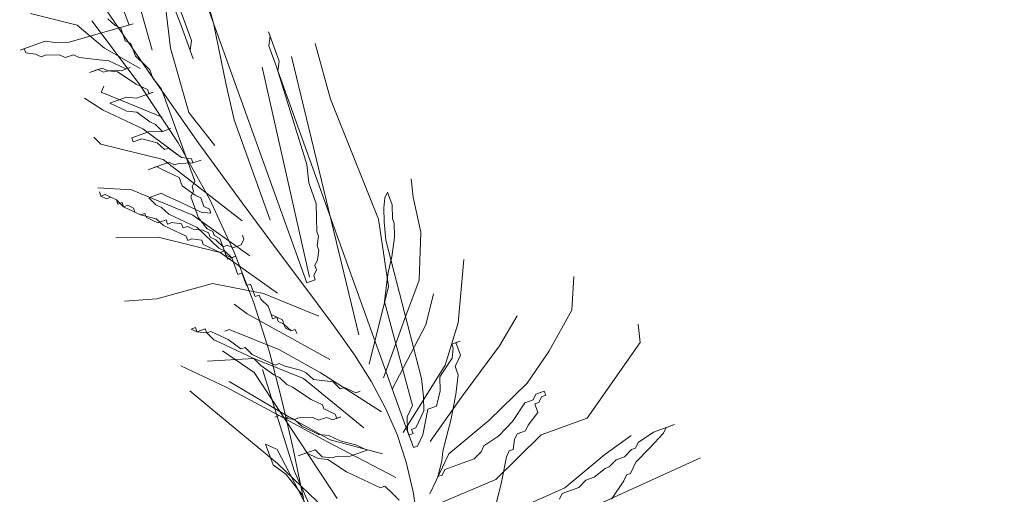
# Model space of a CAD drawing. Units: millimetres. Extents: x 595116 to 630915, y 909473 to 920225.
# Tile 38 of 134: x 629665.643 to 629671.98, y 919177.461 to 919180.516. Entities that reach past the tile are written whole.
import ezdxf

# ---------------------------------------------------------------- set-up
doc = ezdxf.new("R2010")
doc.units = ezdxf.units.MM
doc.layers.add('Dimension', color=3, linetype='Continuous', lineweight=18)
doc.layers.add('L-PLNT', color=85, linetype='Continuous', lineweight=13)
doc.styles.get("Standard").update_dxf_attribs({"font": 'arial.ttf'})
doc.dimstyles.new('ISO-25', dxfattribs={"dimtxt": 9, "dimasz": 6, "dimexe": 1.25, "dimexo": 0.625, "dimtad": 1, "dimlunit": 4, "dimtxsty": 'Standard', "dimcen": 2.5, "dimadec": 0, "dimazin": 0, "dimtfac": 1, "dimtmove": 0, "dimatfit": 3, "dimfxl": 1, "dimarcsym": 0})

# ---------------------------------------------------------------- blocks, each defined once
blk = doc.blocks.new('A$C4FB75ABC')
for p, q in [((2.6279, 3.8295), (2.3336, 4.6475)), ((2.4125, 4.2707), (2.3227, 4.4977)), ((2.3232, 4.271), (2.2922, 4.3571)), ((2.4678, 4.2744), (2.4414, 4.3703)), ((2.2538, 4.3417), (2.3557, 4.1924)), ((2.3628, 4.2285), (2.3338, 4.3316)), ((2.3941, 4.2317), (2.382, 4.3327)), ((2.234, 4.2713), (2.154, 4.2911)), ((2.4119, 4.2948), (2.43, 4.2446)), ((2.2202, 4.242), (2.3304, 4.2736)), ((2.2808, 4.2314), (2.234, 4.2713)), ((2.3407, 4.1707), (2.2593, 4.2788)), ((2.2868, 4.2822), (2.2991, 4.2704)), ((2.4896, 4.1688), (2.4678, 4.2744)), ((2.2991, 4.2704), (2.3089, 4.2658)), ((2.3089, 4.2658), (2.3166, 4.2443)), ((2.4331, 4.2133), (2.4125, 4.2707)), ((2.5803, 4.2095), (2.5622, 4.2597)), ((2.5622, 4.2597), (2.5648, 4.2526)), ((2.1362, 4.228), (2.1792, 4.2435)), ((2.1792, 4.2435), (2.1961, 4.2415)), ((2.1961, 4.2415), (2.2202, 4.242)), ((2.3166, 4.2443), (2.3264, 4.2397)), ((2.3264, 4.2397), (2.3341, 4.2182)), ((2.43, 4.2446), (2.4279, 4.2276)), ((2.5648, 4.2526), (2.5628, 4.2356)), ((2.6686, 4.144), (2.6423, 4.2399)), ((2.1434, 4.2306), (2.1362, 4.228)), ((2.1459, 4.2234), (2.1434, 4.2306)), ((2.1629, 4.2214), (2.1459, 4.2234)), ((2.1726, 4.2168), (2.1629, 4.2214)), ((2.3419, 4.1967), (2.2808, 4.2314)), ((2.4257, 4.1214), (2.3941, 4.2317)), ((2.4279, 4.2276), (2.4331, 4.2133)), ((2.5628, 4.2356), (2.5757, 4.1997)), ((2.1798, 4.2194), (2.1726, 4.2168)), ((2.2039, 4.22), (2.1798, 4.2194)), ((2.2136, 4.2154), (2.2039, 4.22)), ((2.228, 4.2205), (2.2136, 4.2154)), ((2.2377, 4.2159), (2.228, 4.2205)), ((2.2716, 4.2119), (2.2377, 4.2159)), ((2.2885, 4.2099), (2.2716, 4.2119)), ((2.308, 4.2007), (2.2885, 4.2099)), ((2.3341, 4.2182), (2.3465, 4.2064)), ((2.3465, 4.2064), (2.3588, 4.1946)), ((2.5783, 4.1926), (2.5803, 4.2095)), ((2.7169, 3.7399), (2.6018, 4.2172)), ((2.2552, 4.1898), (2.2768, 4.1975)), ((2.2696, 4.195), (2.2552, 4.1898)), ((2.2793, 4.1904), (2.2696, 4.195)), ((2.2768, 4.1975), (2.2865, 4.1929)), ((2.2865, 4.1929), (2.2793, 4.1904)), ((2.2865, 4.1929), (2.3106, 4.1935)), ((2.3034, 4.1909), (2.2865, 4.1929)), ((2.3353, 4.17), (2.3034, 4.1909)), ((2.3178, 4.1961), (2.308, 4.2007)), ((2.3106, 4.1935), (2.325, 4.1987)), ((2.325, 4.1987), (2.3178, 4.1961)), ((2.3557, 4.1924), (2.443, 4.0685)), ((2.3588, 4.1946), (2.364, 4.1803)), ((2.6325, 3.8393), (2.5516, 4.1992)), ((2.5757, 4.1997), (2.6279, 4.0321)), ((2.8029, 3.5683), (2.5783, 4.1926)), ((2.345, 4.1654), (2.3353, 4.17)), ((2.4072, 4.0691), (2.3407, 4.1707)), ((2.364, 4.1803), (2.3789, 4.1614)), ((2.2753, 4.1565), (2.2799, 4.1663)), ((2.38, 4.1131), (2.2753, 4.1565)), ((2.3359, 4.1459), (2.3645, 4.1562)), ((2.3548, 4.1608), (2.345, 4.1654)), ((2.3574, 4.1536), (2.3548, 4.1608)), ((2.3645, 4.1562), (2.3574, 4.1536)), ((2.3789, 4.1614), (2.4357, 4.0035)), ((2.5031, 4.1088), (2.4896, 4.1688)), ((2.2785, 4.1252), (2.2466, 4.1462)), ((2.2902, 4.1376), (2.3189, 4.1479)), ((2.3, 4.133), (2.2902, 4.1376)), ((2.3189, 4.1479), (2.3359, 4.1459)), ((2.7507, 3.9385), (2.6686, 4.144)), ((2.3468, 4.0931), (2.2785, 4.1252)), ((2.3098, 4.1284), (2.3, 4.133)), ((2.3195, 4.1238), (2.3098, 4.1284)), ((2.3364, 4.1218), (2.3195, 4.1238)), ((2.3585, 4.1054), (2.3364, 4.1218)), ((2.4704, 4.0646), (2.4257, 4.1214)), ((2.3683, 4.1008), (2.3585, 4.1054)), ((2.5651, 3.9366), (2.5031, 4.1088)), ((2.3278, 4.0781), (2.3565, 4.0885)), ((2.413, 4.044), (2.3468, 4.0931)), ((2.3565, 4.0885), (2.3806, 4.089)), ((2.3806, 4.089), (2.3683, 4.1008)), ((2.3806, 4.089), (2.395, 4.0942)), ((2.395, 4.0942), (2.3806, 4.089)), ((2.275, 4.0672), (2.2627, 4.079)), ((2.3304, 4.071), (2.3278, 4.0781)), ((2.3448, 4.0761), (2.3304, 4.071)), ((2.3714, 4.0695), (2.3448, 4.0761)), ((2.3838, 4.0577), (2.3714, 4.0695)), ((2.4608, 3.9732), (2.4072, 4.0691)), ((2.3818, 4.0408), (2.275, 4.0672)), ((2.3909, 4.0603), (2.3838, 4.0577)), ((2.413, 4.044), (2.3909, 4.0603)), ((2.443, 4.0685), (2.5171, 3.9664)), ((2.3557, 4.0233), (2.3915, 4.0362)), ((2.5169, 3.9354), (2.3818, 4.0408)), ((2.3915, 4.0362), (2.4013, 4.0316)), ((2.43, 4.0419), (2.413, 4.044)), ((2.4325, 4.0348), (2.43, 4.0419)), ((2.4325, 4.0348), (2.4469, 4.0399)), ((2.4469, 4.0399), (2.4325, 4.0348)), ((2.37, 4.0285), (2.3557, 4.0233)), ((2.3798, 4.0239), (2.37, 4.0285)), ((2.3993, 4.0147), (2.3798, 4.0239)), ((2.4013, 4.0316), (2.4084, 4.0342)), ((2.4084, 4.0342), (2.4325, 4.0348)), ((2.6279, 4.0321), (2.6311, 4.0008)), ((2.409, 4.0101), (2.3993, 4.0147)), ((2.4142, 3.9957), (2.409, 4.0101)), ((2.4357, 4.0035), (2.4311, 3.9937)), ((2.8101, 3.9761), (2.8069, 4.0074)), ((2.3275, 3.9889), (2.2696, 3.9923)), ((2.2748, 3.978), (2.2722, 3.9852)), ((2.2722, 3.9852), (2.2748, 3.978)), ((2.4323, 3.9455), (2.3275, 3.9889)), ((2.4363, 3.9794), (2.4142, 3.9957)), ((2.4337, 3.9866), (2.4291, 3.9768)), ((2.4311, 3.9937), (2.4337, 3.9866)), ((2.6311, 4.0008), (2.644, 3.965)), ((2.7665, 3.9847), (2.7619, 3.975)), ((2.7742, 3.9632), (2.7665, 3.9847)), ((2.2748, 3.978), (2.2819, 3.9806)), ((2.2845, 3.9734), (2.2748, 3.978)), ((2.2819, 3.9806), (2.2917, 3.976)), ((2.2917, 3.976), (2.2845, 3.9734)), ((2.3014, 3.9714), (2.2917, 3.976)), ((2.2917, 3.976), (2.3014, 3.9714)), ((2.304, 3.9642), (2.3014, 3.9714)), ((2.3014, 3.9714), (2.3138, 3.9596)), ((2.3568, 3.9751), (2.3783, 3.9828)), ((2.3691, 3.9633), (2.3568, 3.9751)), ((2.3783, 3.9828), (2.3881, 3.9782)), ((2.3881, 3.9782), (2.4076, 3.9691)), ((2.4076, 3.9691), (2.4173, 3.9645)), ((2.4291, 3.9768), (2.442, 3.9409)), ((2.446, 3.9748), (2.4363, 3.9794)), ((2.4512, 3.9604), (2.446, 3.9748)), ((2.5035, 3.8821), (2.4608, 3.9732)), ((2.7619, 3.975), (2.7599, 3.958)), ((2.8236, 3.9161), (2.8101, 3.9761)), ((2.3112, 3.9668), (2.304, 3.9642)), ((2.3138, 3.9596), (2.3112, 3.9668)), ((2.3209, 3.9622), (2.3138, 3.9596)), ((2.3138, 3.9596), (2.3235, 3.955)), ((2.3307, 3.9576), (2.3209, 3.9622)), ((2.3235, 3.955), (2.3333, 3.9504)), ((2.3333, 3.9504), (2.3307, 3.9576)), ((2.3789, 3.9587), (2.3691, 3.9633)), ((2.3912, 3.947), (2.3789, 3.9587)), ((2.4173, 3.9645), (2.4368, 3.9553)), ((2.4368, 3.9553), (2.4466, 3.9507)), ((2.4466, 3.9507), (2.4635, 3.9487)), ((2.4609, 3.9558), (2.4512, 3.9604)), ((2.4635, 3.9487), (2.4609, 3.9558)), ((2.5171, 3.9664), (2.5794, 3.8826)), ((2.644, 3.965), (2.6451, 3.9167)), ((2.7599, 3.958), (2.7605, 3.9339)), ((2.7748, 3.9391), (2.7742, 3.9632)), ((2.343, 3.9458), (2.3333, 3.9504)), ((2.3333, 3.9504), (2.343, 3.9458)), ((2.3502, 3.9484), (2.343, 3.9458)), ((2.343, 3.9458), (2.3697, 3.9392)), ((2.3528, 3.9412), (2.3502, 3.9484)), ((2.3723, 3.932), (2.3528, 3.9412)), ((2.3697, 3.9392), (2.3821, 3.9274)), ((2.3866, 3.9372), (2.3723, 3.932)), ((2.3892, 3.93), (2.3866, 3.9372)), ((2.401, 3.9424), (2.3912, 3.947)), ((2.44, 3.924), (2.401, 3.9424)), ((2.5304, 3.8755), (2.4323, 3.9455)), ((2.442, 3.9409), (2.4569, 3.922)), ((2.7679, 3.8231), (2.7507, 3.9385)), ((2.7605, 3.9339), (2.7636, 3.9026)), ((2.7774, 3.9319), (2.7748, 3.9391)), ((2.3821, 3.9274), (2.3918, 3.9228)), ((2.3964, 3.9326), (2.3892, 3.93)), ((2.3918, 3.9228), (2.4113, 3.9137)), ((2.4133, 3.9306), (2.3964, 3.9326)), ((2.4159, 3.9234), (2.4133, 3.9306)), ((2.4231, 3.926), (2.4159, 3.9234)), ((2.4328, 3.9214), (2.4231, 3.926)), ((2.4498, 3.9194), (2.4328, 3.9214)), ((2.4523, 3.9122), (2.44, 3.924)), ((2.4595, 3.9148), (2.4498, 3.9194)), ((2.4569, 3.922), (2.4667, 3.9174)), ((2.4667, 3.9174), (2.4693, 3.9102)), ((2.6451, 3.9167), (2.6477, 3.9096)), ((2.778, 3.9078), (2.7774, 3.9319)), ((2.3729, 3.9079), (2.3006, 3.9062)), ((2.4796, 3.8815), (2.3729, 3.9079)), ((2.4113, 3.9137), (2.4211, 3.9091)), ((2.4211, 3.9091), (2.4237, 3.9019)), ((2.4237, 3.9019), (2.4308, 3.9045)), ((2.4308, 3.9045), (2.4478, 3.9025)), ((2.4478, 3.9025), (2.4503, 3.8953)), ((2.477, 3.8887), (2.4523, 3.9122)), ((2.4621, 3.9076), (2.4595, 3.9148)), ((2.4718, 3.903), (2.4621, 3.9076)), ((2.4693, 3.9102), (2.479, 3.9056)), ((2.4842, 3.8913), (2.4718, 3.903)), ((2.479, 3.9056), (2.4868, 3.8841)), ((2.52, 3.9042), (2.5155, 3.8944)), ((2.5175, 3.9113), (2.52, 3.9042)), ((2.6477, 3.9096), (2.6457, 3.8926)), ((2.7636, 3.9026), (2.8247, 3.6653)), ((2.7739, 3.8739), (2.778, 3.9078)), ((2.8207, 3.834), (2.8236, 3.9161)), ((2.4503, 3.8953), (2.4698, 3.8861)), ((2.4698, 3.8861), (2.4796, 3.8815)), ((2.4868, 3.8841), (2.477, 3.8887)), ((2.4796, 3.8815), (2.4868, 3.8841)), ((2.4914, 3.8938), (2.4842, 3.8913)), ((2.4868, 3.8841), (2.4893, 3.8769)), ((2.4919, 3.8697), (2.4868, 3.8841)), ((2.4868, 3.8841), (2.4991, 3.8723)), ((2.5011, 3.8892), (2.4914, 3.8938)), ((2.5155, 3.8944), (2.5011, 3.8892)), ((2.6457, 3.8926), (2.6483, 3.8855)), ((2.6483, 3.8855), (2.6463, 3.8685)), ((2.5777, 3.8114), (2.4796, 3.8815)), ((2.4893, 3.8769), (2.4991, 3.8723)), ((2.5063, 3.8749), (2.4919, 3.8697)), ((2.4991, 3.8723), (2.5063, 3.8749)), ((2.4991, 3.8723), (2.5094, 3.8436)), ((2.5372, 3.7949), (2.5035, 3.8821)), ((2.5794, 3.8826), (2.6314, 3.8136)), ((2.6463, 3.8685), (2.6417, 3.8588)), ((2.7673, 3.8473), (2.7739, 3.8739)), ((2.8876, 3.7608), (2.897, 3.8696)), ((2.6443, 3.8516), (2.6397, 3.8418)), ((2.6417, 3.8588), (2.6443, 3.8516)), ((2.5094, 3.8436), (2.5166, 3.8462)), ((2.5166, 3.8462), (2.5244, 3.8247)), ((2.6423, 3.8347), (2.6279, 3.8295)), ((2.6397, 3.8418), (2.6423, 3.8347)), ((2.7653, 3.8303), (2.7673, 3.8473)), ((2.7957, 3.7683), (2.8207, 3.834)), ((3.0823, 3.7823), (3.0858, 3.8403)), ((2.4664, 3.8281), (2.3706, 3.8017)), ((2.5536, 3.8109), (2.4664, 3.8281)), ((2.5244, 3.8247), (2.5315, 3.8272)), ((2.5315, 3.8272), (2.5393, 3.8057)), ((2.7349, 3.6897), (2.7679, 3.8231)), ((2.7613, 3.7965), (2.7653, 3.8303)), ((2.3706, 3.8017), (2.3152, 3.798)), ((2.5393, 3.8057), (2.5464, 3.8083)), ((2.5464, 3.8083), (2.549, 3.8011)), ((2.549, 3.8011), (2.5614, 3.7893)), ((2.6486, 3.7721), (2.5536, 3.8109)), ((2.6314, 3.8136), (2.6743, 3.7558)), ((2.8322, 3.7571), (2.8454, 3.8105)), ((2.5255, 3.7764), (2.5034, 3.7928)), ((2.5638, 3.7106), (2.5372, 3.7949)), ((2.5614, 3.7893), (2.5665, 3.775)), ((2.8089, 3.6191), (2.7613, 3.7965)), ((3.043, 3.7114), (3.0823, 3.7823)), ((2.6672, 3.6978), (2.5255, 3.7764)), ((2.5665, 3.775), (2.5763, 3.7704)), ((2.5691, 3.7678), (2.5665, 3.775)), ((2.5763, 3.7704), (2.5691, 3.7678)), ((2.5763, 3.7704), (2.5789, 3.7632)), ((2.586, 3.7658), (2.5763, 3.7704)), ((2.5886, 3.7586), (2.586, 3.7658)), ((2.7596, 3.6662), (2.7957, 3.7683)), ((2.9584, 3.7215), (2.9885, 3.7729)), ((2.4369, 3.7526), (2.4297, 3.7501)), ((2.4297, 3.7501), (2.4394, 3.7455)), ((2.4394, 3.7455), (2.4369, 3.7526)), ((2.4538, 3.7506), (2.4394, 3.7455)), ((2.4564, 3.7435), (2.4538, 3.7506)), ((2.4948, 3.7492), (2.4876, 3.7466)), ((2.58, 3.715), (2.4948, 3.7492)), ((2.5789, 3.7632), (2.5886, 3.7586)), ((2.5886, 3.7586), (2.5912, 3.7515)), ((2.601, 3.7469), (2.5886, 3.7586)), ((2.5912, 3.7515), (2.601, 3.7469)), ((2.601, 3.7469), (2.6081, 3.7494)), ((2.6081, 3.7494), (2.601, 3.7469)), ((2.6081, 3.7494), (2.6107, 3.7423)), ((2.6107, 3.7423), (2.6081, 3.7494)), ((2.6743, 3.7558), (2.7096, 3.7056)), ((2.7745, 3.6472), (2.8322, 3.7571)), ((2.8652, 3.6879), (2.8876, 3.7608)), ((3.1994, 3.7272), (3.1962, 3.7584)), ((2.4394, 3.7455), (2.4564, 3.7435)), ((2.4635, 3.746), (2.4564, 3.7435)), ((2.4564, 3.7435), (2.4687, 3.7317)), ((2.4733, 3.7414), (2.4635, 3.746)), ((2.4687, 3.7317), (2.4785, 3.7271)), ((2.4928, 3.7323), (2.4733, 3.7414)), ((2.5149, 3.7159), (2.4928, 3.7323)), ((2.4785, 3.7271), (2.498, 3.7179)), ((2.498, 3.7179), (2.5272, 3.7041)), ((2.5221, 3.7185), (2.5149, 3.7159)), ((2.5344, 3.7067), (2.5221, 3.7185)), ((2.6509, 3.6757), (2.58, 3.715)), ((2.8907, 3.7295), (2.8764, 3.7244)), ((2.8764, 3.7244), (2.8789, 3.7172)), ((2.8789, 3.7172), (2.8769, 3.7003)), ((2.8835, 3.727), (2.8907, 3.7295)), ((2.8913, 3.7054), (2.8835, 3.727)), ((2.893, 3.6331), (2.9584, 3.7215)), ((3.1085, 3.5972), (3.1994, 3.7272)), ((2.537, 3.6995), (2.4575, 3.6952)), ((2.5376, 3.6754), (2.4836, 3.7127)), ((2.5272, 3.7041), (2.537, 3.6995)), ((2.5441, 3.7021), (2.5344, 3.7067)), ((2.537, 3.6995), (2.5493, 3.6877)), ((2.6222, 3.6653), (2.537, 3.6995)), ((2.5637, 3.6929), (2.5441, 3.7021)), ((2.5853, 3.6284), (2.5638, 3.7106)), ((2.7096, 3.7056), (2.7388, 3.6597)), ((2.8769, 3.7003), (2.856, 3.6684)), ((2.8821, 3.6859), (2.8913, 3.7054)), ((3.0058, 3.6575), (3.043, 3.7114)), ((2.4899, 3.6502), (2.4119, 3.6869)), ((2.5493, 3.6877), (2.5714, 3.6714)), ((2.6067, 3.5058), (2.5519, 3.6806)), ((2.5734, 3.6883), (2.5637, 3.6929)), ((2.5806, 3.6909), (2.5734, 3.6883)), ((2.5903, 3.6863), (2.5806, 3.6909)), ((2.617, 3.6797), (2.5903, 3.6863)), ((2.7932, 3.5729), (2.8652, 3.6879)), ((2.8873, 3.6716), (2.8821, 3.6859)), ((2.6801, 3.4593), (2.5376, 3.6754)), ((2.5714, 3.6714), (2.5812, 3.6668)), ((2.5812, 3.6668), (2.5935, 3.655)), ((2.6268, 3.6751), (2.617, 3.6797)), ((2.7255, 3.5809), (2.6222, 3.6653)), ((2.6391, 3.6633), (2.6268, 3.6751)), ((2.7562, 3.6082), (2.6509, 3.6757)), ((2.8247, 3.6653), (2.8279, 3.634)), ((2.856, 3.6684), (2.8566, 3.6443)), ((2.8833, 3.6377), (2.8873, 3.6716)), ((2.5803, 3.6016), (2.4899, 3.6502)), ((2.5972, 3.5996), (2.4945, 3.6599)), ((2.5935, 3.655), (2.6032, 3.6504)), ((2.6032, 3.6504), (2.6351, 3.6295)), ((2.673, 3.6593), (2.6391, 3.6633)), ((2.6853, 3.6475), (2.673, 3.6593)), ((2.6925, 3.6501), (2.6853, 3.6475)), ((2.7022, 3.6455), (2.6925, 3.6501)), ((2.7388, 3.6597), (2.763, 3.6147)), ((2.9398, 3.5932), (3.0058, 3.6575)), ((2.4618, 3.6157), (2.4274, 3.6439)), ((2.712, 3.6409), (2.7022, 3.6455)), ((2.7192, 3.6435), (2.712, 3.6409)), ((2.8279, 3.634), (2.8285, 3.6099)), ((2.8394, 3.5571), (2.893, 3.6331)), ((2.8566, 3.6443), (2.85, 3.6176)), ((2.8746, 3.5941), (2.8833, 3.6377)), ((3.0207, 3.6385), (3.0161, 3.6288)), ((3.035, 3.6437), (3.0207, 3.6385)), ((3.0258, 3.6242), (3.0304, 3.6339)), ((3.0304, 3.6339), (3.0376, 3.6365)), ((3.0376, 3.6365), (3.035, 3.6437)), ((2.5774, 3.5196), (2.4618, 3.6157)), ((2.6037, 3.5475), (2.5853, 3.6284)), ((2.6351, 3.6295), (2.6448, 3.6249)), ((2.6448, 3.6249), (2.6546, 3.6203)), ((2.6546, 3.6203), (2.6572, 3.6131)), ((2.6572, 3.6131), (2.6669, 3.6085)), ((2.763, 3.6147), (2.7827, 3.5691)), ((2.7998, 3.5996), (2.8089, 3.6191)), ((2.85, 3.6176), (2.8356, 3.6125)), ((3.0017, 3.6236), (2.9808, 3.5918)), ((3.0161, 3.6288), (3.0017, 3.6236)), ((3.0187, 3.6216), (3.0258, 3.6242)), ((3.0238, 3.6072), (3.0187, 3.6216)), ((2.5803, 3.6016), (2.5731, 3.5991)), ((2.5731, 3.5991), (2.5803, 3.6016)), ((2.5901, 3.597), (2.5803, 3.6016)), ((2.5803, 3.6016), (2.5901, 3.597)), ((2.6609, 3.5577), (2.5803, 3.6016)), ((2.5972, 3.5996), (2.5901, 3.597)), ((2.5901, 3.597), (2.607, 3.595)), ((2.607, 3.595), (2.5972, 3.5996)), ((2.6681, 3.5603), (2.5972, 3.5996)), ((2.6142, 3.5976), (2.607, 3.595)), ((2.6383, 3.5982), (2.6142, 3.5976)), ((2.648, 3.5936), (2.6383, 3.5982)), ((2.6623, 3.5987), (2.648, 3.5936)), ((2.6721, 3.5942), (2.6623, 3.5987)), ((2.6669, 3.6085), (2.6767, 3.6039)), ((2.6864, 3.5993), (2.6721, 3.5942)), ((2.6767, 3.6039), (2.6793, 3.5967)), ((2.6793, 3.5967), (2.6864, 3.5993)), ((2.8003, 3.5755), (2.7998, 3.5996)), ((2.8285, 3.6099), (2.8193, 3.5904)), ((2.8356, 3.6125), (2.827, 3.5688)), ((3.0075, 3.5852), (3.0238, 3.6072)), ((3.0296, 3.5688), (3.1085, 3.5972)), ((2.607, 3.595), (2.6193, 3.5833)), ((2.6193, 3.5833), (2.6486, 3.5695)), ((2.8147, 3.5806), (2.8075, 3.578)), ((2.8193, 3.5904), (2.8147, 3.5806)), ((2.868, 3.5674), (2.8746, 3.5941)), ((2.8712, 3.5361), (2.9398, 3.5932)), ((2.969, 3.5794), (2.9573, 3.5671)), ((2.9808, 3.5918), (2.969, 3.5794)), ((3.0029, 3.5754), (3.0075, 3.5852)), ((3.2582, 3.5862), (3.2224, 3.5733)), ((3.2393, 3.5713), (3.2439, 3.5811)), ((3.2439, 3.5811), (3.2582, 3.5862)), ((2.6486, 3.5695), (2.6655, 3.5675)), ((2.6655, 3.5675), (2.685, 3.5583)), ((2.7827, 3.5691), (2.7983, 3.5216)), ((2.8107, 3.5468), (2.8003, 3.5755)), ((2.8101, 3.5709), (2.8029, 3.5683)), ((2.8075, 3.578), (2.8101, 3.5709)), ((2.827, 3.5688), (2.8224, 3.5591)), ((2.8614, 3.5407), (2.868, 3.5674)), ((2.9573, 3.5671), (2.9312, 3.5496)), ((2.9518, 3.4922), (3.0296, 3.5688)), ((2.984, 3.5605), (2.9885, 3.5702)), ((2.9885, 3.5702), (3.0029, 3.5754)), ((3.1389, 3.5352), (3.1839, 3.5676)), ((3.2224, 3.5733), (3.1962, 3.5558)), ((3.2158, 3.5466), (3.2393, 3.5713)), ((2.5671, 3.5483), (2.5573, 3.5529)), ((2.5573, 3.5529), (2.5703, 3.517)), ((2.5769, 3.5437), (2.5671, 3.5483)), ((2.6204, 3.467), (2.6037, 3.5475)), ((2.7805, 3.4954), (2.6609, 3.5577)), ((2.7579, 3.5359), (2.6681, 3.5603)), ((2.685, 3.5583), (2.7117, 3.5517)), ((2.7117, 3.5517), (2.7214, 3.5471)), ((2.7214, 3.5471), (2.7312, 3.5425)), ((2.8178, 3.5493), (2.8107, 3.5468)), ((2.8224, 3.5591), (2.8178, 3.5493)), ((2.9312, 3.5496), (2.9266, 3.5398)), ((2.9819, 3.5435), (2.984, 3.5605)), ((3.1917, 3.5461), (3.1845, 3.5435)), ((3.1962, 3.5558), (3.1917, 3.5461)), ((3.1922, 3.522), (3.2158, 3.5466)), ((2.6552, 3.3935), (2.5769, 3.5437)), ((2.642, 3.5428), (2.6133, 3.5325)), ((2.6133, 3.5325), (2.6276, 3.5376)), ((2.6276, 3.5376), (2.6471, 3.5284)), ((2.6543, 3.531), (2.642, 3.5428)), ((2.6471, 3.5284), (2.6641, 3.5264)), ((2.6712, 3.529), (2.6543, 3.531)), ((2.6784, 3.5316), (2.6712, 3.529)), ((2.7025, 3.5321), (2.6784, 3.5316)), ((2.7312, 3.5425), (2.7025, 3.5321)), ((2.8391, 3.4678), (2.8712, 3.5361)), ((2.8594, 3.5238), (2.8614, 3.5407)), ((2.9266, 3.5398), (2.9148, 3.5275)), ((2.9616, 3.4876), (2.9702, 3.5312)), ((2.9702, 3.5312), (2.9748, 3.541)), ((2.9748, 3.541), (2.9819, 3.5435)), ((3.0703, 3.4781), (3.1389, 3.5352)), ((3.136, 3.4531), (3.303, 3.5294)), ((3.1727, 3.5311), (3.1584, 3.526)), ((3.1845, 3.5435), (3.1727, 3.5311)), ((2.5703, 3.517), (2.5924, 3.5006)), ((2.6885, 3.4136), (2.5774, 3.5196)), ((2.6641, 3.5264), (2.6959, 3.5055)), ((2.7983, 3.5216), (2.81, 3.4712)), ((2.8528, 3.4971), (2.8594, 3.5238)), ((2.9148, 3.5275), (2.8646, 3.5094)), ((3.1466, 3.5136), (3.1394, 3.5111)), ((3.1584, 3.526), (3.1466, 3.5136)), ((3.1831, 3.5024), (3.1922, 3.522)), ((2.5924, 3.5006), (2.6222, 3.4627)), ((2.7237, 3.248), (2.6067, 3.5058)), ((2.6959, 3.5055), (2.7154, 3.4963)), ((2.7154, 3.4963), (2.7252, 3.4917)), ((2.86, 3.4997), (2.8528, 3.4971)), ((2.8646, 3.5094), (2.86, 3.4997)), ((3.1205, 3.4961), (3.1062, 3.491)), ((3.1394, 3.5111), (3.1205, 3.4961)), ((3.1713, 3.4901), (3.1759, 3.4999)), ((3.1759, 3.4999), (3.1831, 3.5024)), ((2.7252, 3.4917), (2.7544, 3.4779)), ((2.7544, 3.4779), (2.7616, 3.4805)), ((2.7616, 3.4805), (2.774, 3.4687)), ((2.8253, 3.4385), (2.9518, 3.4922)), ((2.9484, 3.4342), (2.9616, 3.4876)), ((2.9797, 3.4374), (3.0703, 3.4781)), ((3.0944, 3.4786), (3.0657, 3.4683)), ((3.1062, 3.491), (3.0944, 3.4786)), ((3.1503, 3.4583), (3.1713, 3.4901)), ((2.636, 3.3873), (2.6204, 3.467)), ((2.774, 3.4687), (2.7863, 3.4569)), ((2.81, 3.4712), (2.8183, 3.4166)), ((3.0657, 3.4683), (3.0611, 3.4586))]:
    blk.add_line(p, q)
blk = doc.blocks.new('*D216')
at = {"layer": 'Defpoints', "color": 0, "transparency": 16777216}
for p in [(629743.5408, 919411.9276), (629505.0408, 919411.8279), (629743.5408, 918832.3776)]:
    blk.add_point(p, dxfattribs=at)
at = {"layer": 'Dimension', "color": 0, "lineweight": -2, "transparency": 16777216}
for p, q in [((629743.5408, 919411.3026), (629743.5408, 918831.1276)), ((629505.0408, 919411.2029), (629505.0408, 918831.1276)), ((629511.0408, 918832.3776), (629737.5408, 918832.3776))]:
    blk.add_line(p, q, dxfattribs=at)
at = {"layer": 'Dimension', "color": 0, "transparency": 16777216}
for points in [[(629511.0408, 918833.3776), (629511.0408, 918831.3776), (629505.0408, 918832.3776)], [(629737.5408, 918833.3776), (629737.5408, 918831.3776), (629743.5408, 918832.3776)]]:
    blk.add_solid(points, dxfattribs=at)
at = {"layer": 'Dimension', "color": 0, "transparency": 16777216, "insert": (629624.2908, 918837.656), "char_height": 9, "attachment_point": 5}
blk.add_mtext('19\'-10 1/2"', dxfattribs=at)

msp = doc.modelspace()

# ---------------------------------------------------------------- block references
at = {"layer": 'L-PLNT', "xscale": 3.753413438031968, "yscale": 3.753413438031968, "zscale": 3.753413438031968}
msp.add_blockref('A$C4FB75ABC', (629657.6275, 919164.4492), dxfattribs=at)

# ---------------------------------------------------------------- dimensions: what is measured, and where the dimension line sits
at = {"layer": 'Dimension'}
dim = msp.add_linear_dim(base=(629743.5408, 918832.3776), p1=(629505.0408, 919411.8279), p2=(629743.5408, 919411.9276), dimstyle='ISO-25', override={"dimdec": 1, "dimlfac": 1, "dimrnd": 0, "dimzin": 1, "dimdsep": 46, "dimlunit": 4, "dimfrac": 2}, dxfattribs=at)
dim.commit()
dim.dimension.update_dxf_attribs({"geometry": '*D216', "text_midpoint": (629624.2908, 918837.656)})

doc.saveas('drawing.dxf')
